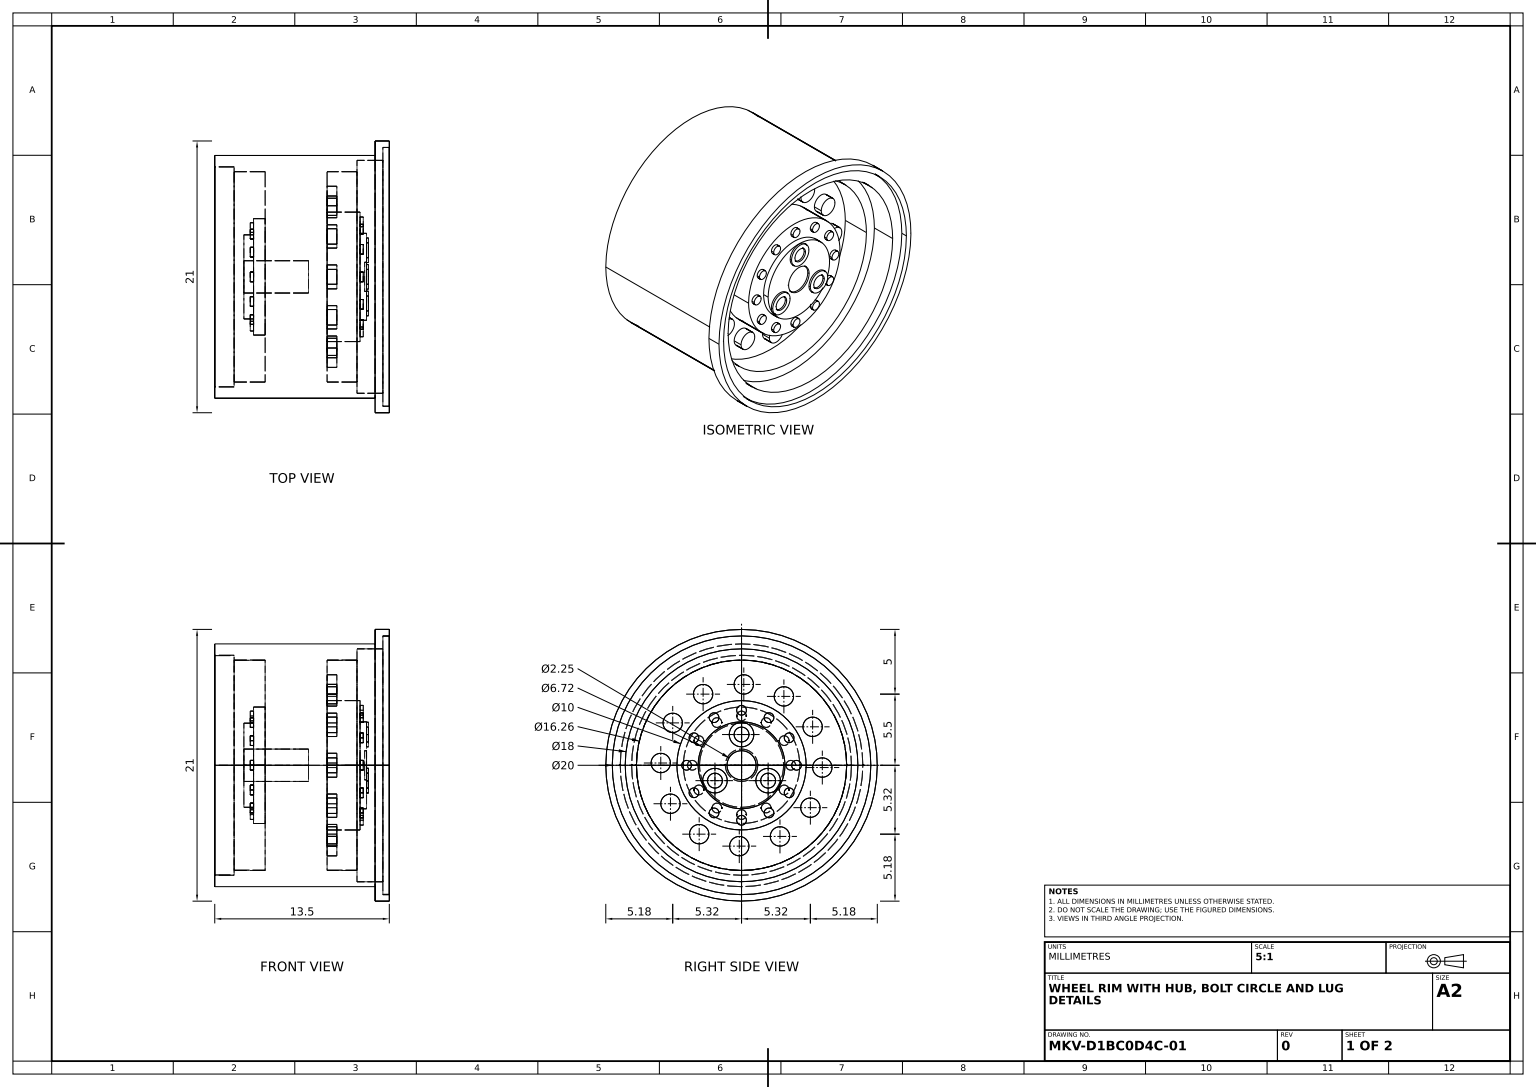
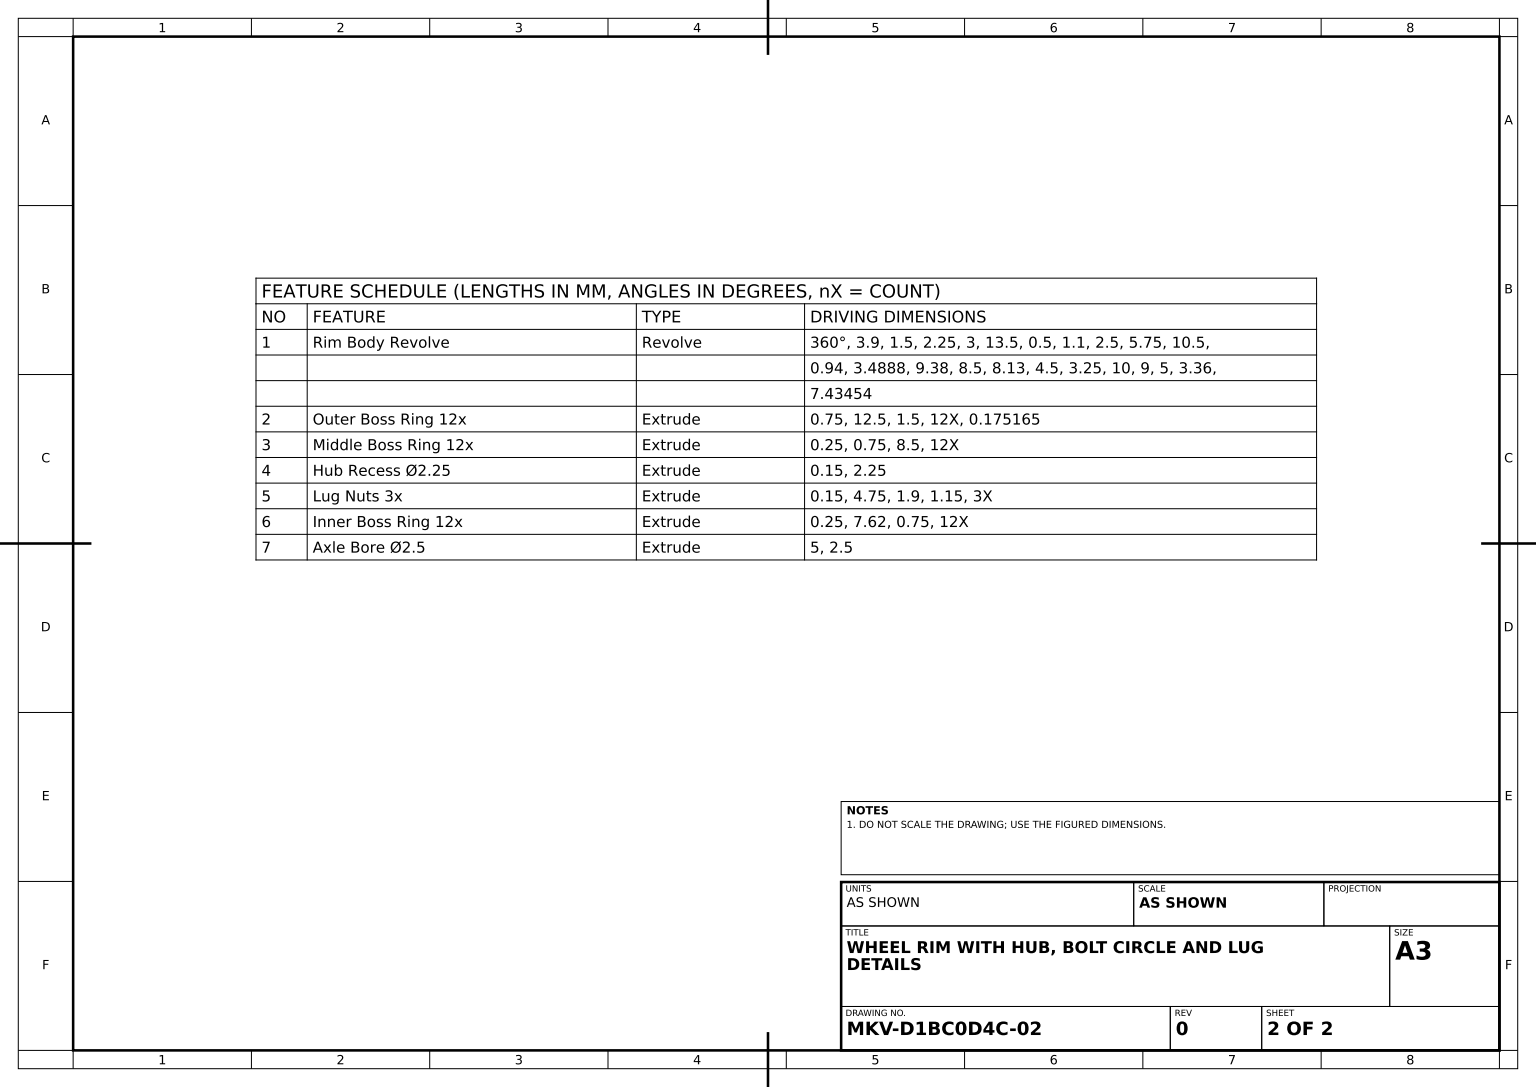
from build123d import *

# Parameters (mm, degrees)
OUTER_BOSS_RING_SKETCH_12X_1_5_R = 0.75
OUTER_BOSS_RING_12X_DEPTH        = 0.75
MIDDLE_BOSS_RING_SKETCH_12X_R    = 0.375
MIDDLE_BOSS_RING_12X_DEPTH       = 0.25
HUB_RECESS_SKETCH_2_25_R         = 1.125
HUB_RECESS_2_25_DEPTH            = 0.15
LUG_NUTS_SKETCH_3X_R             = 0.95
LUG_NUTS_SKETCH_3X_R_2           = 0.575
LUG_NUTS_3X_DEPTH                = 0.15
INNER_BOSS_RING_SKETCH_12X_R     = 0.375
INNER_BOSS_RING_12X_DEPTH        = 0.25
AXLE_BORE_SKETCH_2_5_R           = 1.25
AXLE_BORE_2_5_DEPTH              = 5


with BuildPart() as part:
    # Rim Profile Sketch → Rim Body Revolve (revolve)
    with BuildSketch(Plane.XY, mode=Mode.PRIVATE) as rim_body_revolve_sk:
        Polygon((4.65, 9.38), (0, 9.38), (-7.75, 9.38), (-7.75, 8.5), (-6.25, 8.5), (-6.25, 8.13), (-3.85, 8.13), (-3.85, 4.5), (-4.75, 4.5), (-4.75, 3.25), (-5.5, 3.25), (-5.5, 0), (3.988800196, 0), (3.988800196, 3.36), (3.488800196, 3.36), (3.488800196, 5), (0.94, 5), (0.94, 8.13), (3.25, 8.13), (3.25, 9), (5.25, 9), (5.25, 10), (5.75, 10), (5.75, 10.5), (4.65, 10.5), align=None)
    revolve(rim_body_revolve_sk.sketch.rotate(Axis((0, 0, 0), (1, 0, 0)), 90), axis=Axis((0, 0, 0), (1, 0, 0)))

    # Outer Boss Ring Sketch 12xØ1.5 → Outer Boss Ring 12x (add)
    with BuildSketch(Plane(origin=(0.94, 0, 0), x_dir=(0, 0, -1), z_dir=(1, 0, 0))):
        with Locations((0.17516481, 6.247544901)):
            Circle(OUTER_BOSS_RING_SKETCH_12X_1_5_R)
        with Locations((3.275469626, 5.32295019)):
            Circle(OUTER_BOSS_RING_SKETCH_12X_1_5_R)
        with Locations((5.498115001, 2.972075275)):
            Circle(OUTER_BOSS_RING_SKETCH_12X_1_5_R)
        with Locations((6.247544901, -0.17516481)):
            Circle(OUTER_BOSS_RING_SKETCH_12X_1_5_R)
        with Locations((5.32295019, -3.275469626)):
            Circle(OUTER_BOSS_RING_SKETCH_12X_1_5_R)
        with Locations((2.972075275, -5.498115001)):
            Circle(OUTER_BOSS_RING_SKETCH_12X_1_5_R)
        with Locations((-0.17516481, -6.247544901)):
            Circle(OUTER_BOSS_RING_SKETCH_12X_1_5_R)
        with Locations((-3.275469626, -5.32295019)):
            Circle(OUTER_BOSS_RING_SKETCH_12X_1_5_R)
        with Locations((-5.498115001, -2.972075275)):
            Circle(OUTER_BOSS_RING_SKETCH_12X_1_5_R)
        with Locations((-6.247544901, 0.17516481)):
            Circle(OUTER_BOSS_RING_SKETCH_12X_1_5_R)
        with Locations((-5.32295019, 3.275469626)):
            Circle(OUTER_BOSS_RING_SKETCH_12X_1_5_R)
        with Locations((-2.972075275, 5.498115001)):
            Circle(OUTER_BOSS_RING_SKETCH_12X_1_5_R)
    extrude(amount=OUTER_BOSS_RING_12X_DEPTH)

    # Middle Boss Ring Sketch 12x → Middle Boss Ring 12x (add)
    with BuildSketch(Plane(origin=(3.488800196, 0, 0), x_dir=(0, 0, -1), z_dir=(1, 0, 0))):
        with Locations((0, 4.25)):
            Circle(MIDDLE_BOSS_RING_SKETCH_12X_R)
        with Locations((2.125, 3.680607966)):
            Circle(MIDDLE_BOSS_RING_SKETCH_12X_R)
        with Locations((3.680607966, 2.125)):
            Circle(MIDDLE_BOSS_RING_SKETCH_12X_R)
        with Locations((4.25, 0)):
            Circle(MIDDLE_BOSS_RING_SKETCH_12X_R)
        with Locations((3.680607966, -2.125)):
            Circle(MIDDLE_BOSS_RING_SKETCH_12X_R)
        with Locations((2.125, -3.680607966)):
            Circle(MIDDLE_BOSS_RING_SKETCH_12X_R)
        with Locations((0, -4.25)):
            Circle(MIDDLE_BOSS_RING_SKETCH_12X_R)
        with Locations((-2.125, -3.680607966)):
            Circle(MIDDLE_BOSS_RING_SKETCH_12X_R)
        with Locations((-3.680607966, -2.125)):
            Circle(MIDDLE_BOSS_RING_SKETCH_12X_R)
        with Locations((-4.25, 0)):
            Circle(MIDDLE_BOSS_RING_SKETCH_12X_R)
        with Locations((-3.680607966, 2.125)):
            Circle(MIDDLE_BOSS_RING_SKETCH_12X_R)
        with Locations((-2.125, 3.680607966)):
            Circle(MIDDLE_BOSS_RING_SKETCH_12X_R)
    extrude(amount=MIDDLE_BOSS_RING_12X_DEPTH)

    # Hub Recess Sketch Ø2.25 → Hub Recess Ø2.25 (cut)
    with BuildSketch(Plane(origin=(3.988800196, 0, 0), x_dir=(0, 0, -1), z_dir=(1, 0, 0))):
        Circle(HUB_RECESS_SKETCH_2_25_R)
    extrude(amount=-HUB_RECESS_2_25_DEPTH, mode=Mode.SUBTRACT)

    # Lug Nuts Sketch 3x → Lug Nuts 3x (add)
    # profile 1 of 3: a face of its own
    with BuildSketch(Plane(origin=(3.988800196, 0, 0), x_dir=(0, 0, -1), z_dir=(1, 0, 0))):
        with Locations((0, 2.375)):
            Circle(LUG_NUTS_SKETCH_3X_R)
        with Locations((0, 2.375)):
            Circle(LUG_NUTS_SKETCH_3X_R_2, mode=Mode.SUBTRACT)
    # profile 2 of 3: a face of its own
    with BuildSketch(Plane(origin=(3.988800196, 0, 0), x_dir=(0, 0, -1), z_dir=(1, 0, 0))):
        with Locations((2.056810334, -1.1875)):
            Circle(LUG_NUTS_SKETCH_3X_R)
        with Locations((2.056810334, -1.1875)):
            Circle(LUG_NUTS_SKETCH_3X_R_2, mode=Mode.SUBTRACT)
    # profile 3 of 3: a face of its own
    with BuildSketch(Plane(origin=(3.988800196, 0, 0), x_dir=(0, 0, -1), z_dir=(1, 0, 0))):
        with Locations((-2.056810334, -1.1875)):
            Circle(LUG_NUTS_SKETCH_3X_R)
        with Locations((-2.056810334, -1.1875)):
            Circle(LUG_NUTS_SKETCH_3X_R_2, mode=Mode.SUBTRACT)
    extrude(amount=LUG_NUTS_3X_DEPTH)

    # Inner Boss Ring Sketch 12x → Inner Boss Ring 12x (add)
    with BuildSketch(Plane.ZY.offset(4.75)):
        with Locations(Location((0, 3.81, 0), (0, 0, 180))):
            Circle(INNER_BOSS_RING_SKETCH_12X_R)
        with Locations(Location((1.905, 3.299556788, 0), (0, 0, 180))):
            Circle(INNER_BOSS_RING_SKETCH_12X_R)
        with Locations(Location((3.299556788, 1.905, 0), (0, 0, 180))):
            Circle(INNER_BOSS_RING_SKETCH_12X_R)
        with Locations(Location((3.81, 0, 0), (0, 0, 180))):
            Circle(INNER_BOSS_RING_SKETCH_12X_R)
        with Locations(Location((3.299556788, -1.905, 0), (0, 0, 180))):
            Circle(INNER_BOSS_RING_SKETCH_12X_R)
        with Locations(Location((1.905, -3.299556788, 0), (0, 0, 180))):
            Circle(INNER_BOSS_RING_SKETCH_12X_R)
        with Locations(Location((0, -3.81, 0), (0, 0, 180))):
            Circle(INNER_BOSS_RING_SKETCH_12X_R)
        with Locations(Location((-1.905, -3.299556788, 0), (0, 0, 180))):
            Circle(INNER_BOSS_RING_SKETCH_12X_R)
        with Locations(Location((-3.299556788, -1.905, 0), (0, 0, 180))):
            Circle(INNER_BOSS_RING_SKETCH_12X_R)
        with Locations(Location((-3.81, 0, 0), (0, 0, 180))):
            Circle(INNER_BOSS_RING_SKETCH_12X_R)
        with Locations(Location((-3.299556788, 1.905, 0), (0, 0, 180))):
            Circle(INNER_BOSS_RING_SKETCH_12X_R)
        with Locations(Location((-1.905, 3.299556788, 0), (0, 0, 180))):
            Circle(INNER_BOSS_RING_SKETCH_12X_R)
    extrude(amount=INNER_BOSS_RING_12X_DEPTH)

    # Axle Bore Sketch Ø2.5 → Axle Bore Ø2.5 (cut)
    with BuildSketch(Plane.ZY.offset(5.5)):
        Circle(AXLE_BORE_SKETCH_2_5_R)
    extrude(amount=-AXLE_BORE_2_5_DEPTH, mode=Mode.SUBTRACT)


solid = part.part
